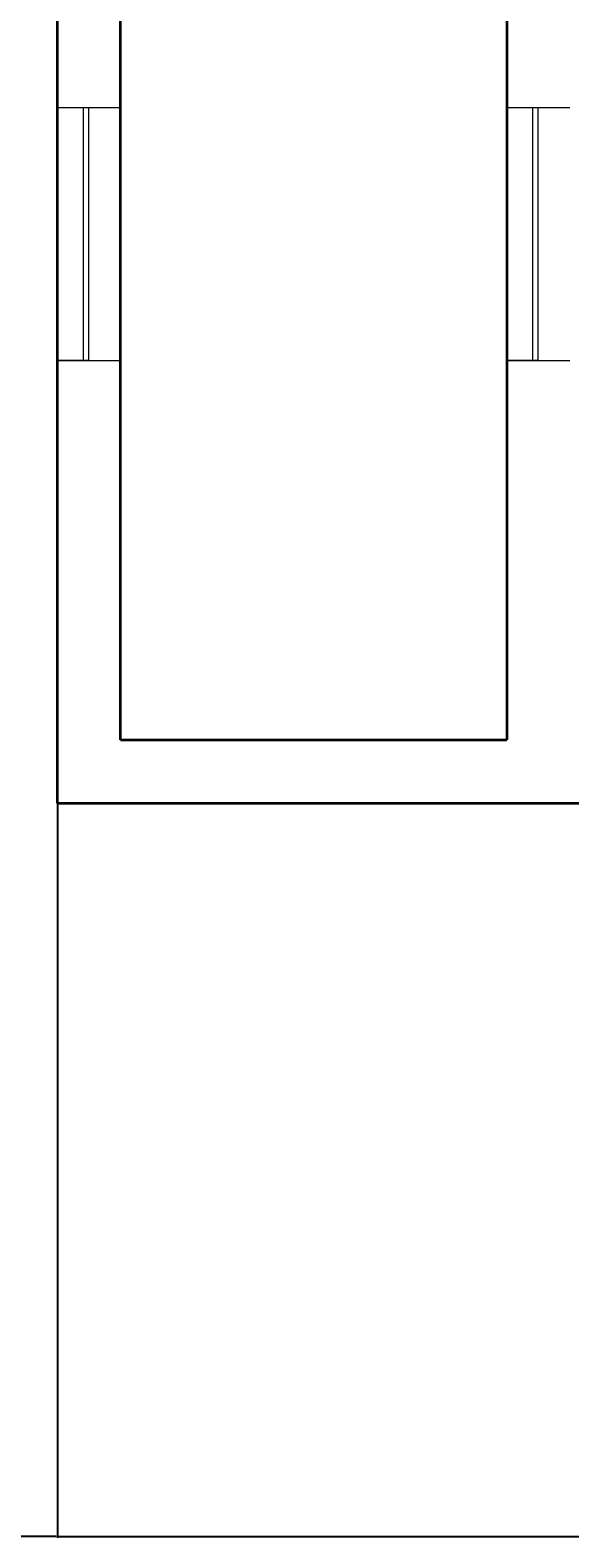
# Model space of a CAD drawing. Units: inches. Extents: x -61 to 1599, y -1316 to 257.
# Tile 156 of 204: x 989 to 1066, y -1316 to -1101. Entities that reach past the tile are written whole.
import ezdxf

# ---------------------------------------------------------------- set-up
doc = ezdxf.new("R2010")
doc.units = ezdxf.units.IN
doc.header["$MEASUREMENT"] = 0
for name, color, linetype, lineweight in [('A-ANNO-DIMS', 2, 'Continuous', 18), ('WALLS', 4, 'Continuous', 35), ('WINDOWS', 220, 'Continuous', 18)]:
    doc.layers.add(name, color=color, linetype=linetype, lineweight=lineweight)
doc.styles.get("Standard").update_dxf_attribs({"font": 'arial.ttf'})
doc.dimstyles.get("Standard").update_dxf_attribs({"dimtxt": 0.18, "dimasz": 0.18, "dimexe": 0.18, "dimexo": 0.0625, "dimgap": 0.09, "dimtad": 0, "dimtih": 1, "dimtoh": 1, "dimdec": 0, "dimzin": 0, "dimdsep": 46, "dimlunit": 3, "dimtxsty": 'Standard', "dimcen": 0.09, "dimadec": 0, "dimazin": 0, "dimtfac": 1, "dimtdec": 0, "dimtofl": 0, "dimtmove": 0, "dimatfit": 3, "dimfxl": 1, "dimtolj": 1, "dimtzin": 0, "dimarcsym": 0})

# ---------------------------------------------------------------- blocks, each defined once
blk = doc.blocks.new('WIN-36IN')
for p, q in [((0, 4.5), (0, 9)), ((0, 9), (0, 0)), ((36, 9), (36, 0)), ((0, 5.26), (36, 5.26)), ((0, 4.5), (36, 4.5)), ((0, 4.5), (36, 4.5))]:
    blk.add_line(p, q)
blk = doc.blocks.new('*D689')
at = {"layer": 'A-ANNO-DIMS', "color": 0, "lineweight": -2, "transparency": 16777216}
for p, q in [((992.7, -1211.23), (992.7, -1315.72)), ((544.7, -1216.01), (544.7, -1315.72)), ((544.88, -1315.54), (768.41, -1315.54)), ((992.52, -1315.54), (769, -1315.54))]:
    blk.add_line(p, q, dxfattribs=at)
at = {"layer": 'A-ANNO-DIMS', "color": 0, "transparency": 16777216}
for points in [[(544.88, -1315.51), (544.88, -1315.57), (544.7, -1315.54)], [(992.52, -1315.51), (992.52, -1315.57), (992.7, -1315.54)]]:
    blk.add_solid(points, dxfattribs=at)
at = {"layer": 'DEFPOINTS', "color": 0, "transparency": 16777216}
for p in [(992.7, -1211.17), (544.7, -1215.94), (992.7, -1315.54)]:
    blk.add_point(p, dxfattribs=at)
at = {"layer": 'A-ANNO-DIMS', "color": 0, "transparency": 16777216, "insert": (768.7, -1315.54), "char_height": 0.18, "attachment_point": 5}
blk.add_mtext('\\A1;448', dxfattribs=at)
blk = doc.blocks.new('*D690')
at = {"layer": 'A-ANNO-DIMS', "color": 0, "lineweight": -2, "transparency": 16777216}
for p, q in [((992.7, -1211.23), (992.7, -1315.72)), ((1522.7, -1211.23), (1522.7, -1315.72)), ((992.88, -1315.54), (1257.41, -1315.54)), ((1522.52, -1315.54), (1257.99, -1315.54))]:
    blk.add_line(p, q, dxfattribs=at)
at = {"layer": 'A-ANNO-DIMS', "color": 0, "transparency": 16777216}
for points in [[(992.88, -1315.51), (992.88, -1315.57), (992.7, -1315.54)], [(1522.52, -1315.51), (1522.52, -1315.57), (1522.7, -1315.54)]]:
    blk.add_solid(points, dxfattribs=at)
at = {"layer": 'DEFPOINTS', "color": 0, "transparency": 16777216}
for p in [(992.7, -1211.17), (1522.7, -1211.17), (1522.7, -1315.54)]:
    blk.add_point(p, dxfattribs=at)
at = {"layer": 'A-ANNO-DIMS', "color": 0, "transparency": 16777216, "insert": (1257.7, -1315.54), "char_height": 0.18, "attachment_point": 5}
blk.add_mtext('\\A1;530', dxfattribs=at)

msp = doc.modelspace()

# ---------------------------------------------------------------- linework, layer by layer
at = {"layer": 'WALLS'}
for p, q in [((992.7028, -1211.169), (992.7028, -741.169)), ((1001.7028, -1202.169), (1001.7028, -777.169)), ((1056.7028, -945.169), (1056.7028, -1202.169)), ((1001.7028, -1202.169), (1056.7028, -1202.169)), ((992.7028, -1211.169), (1215.7028, -1211.169))]:
    msp.add_line(p, q, dxfattribs=at)

# ---------------------------------------------------------------- block references
at = {"layer": 'WINDOWS'}
for p, rotation in [((1001.7029, -1148.1651), 89.99999999999969), ((1065.7029, -1148.1651), 89.99999999999939)]:
    msp.add_blockref('WIN-36IN', p, dxfattribs=dict(at, rotation=rotation))

# ---------------------------------------------------------------- dimensions: what is measured, and where the dimension line sits
at = {"layer": 'A-ANNO-DIMS'}
for base, p1, p2, picture, middle in [((992.7028, -1315.5446), (544.7028, -1215.9446), (992.7028, -1211.169), '*D689', (768.7028, -1315.5446)), ((1522.7028, -1315.5446), (992.7028, -1211.169), (1522.7028, -1211.169), '*D690', (1257.7028, -1315.5446))]:
    dim = msp.add_linear_dim(base=base, p1=p1, p2=p2, dimstyle='Standard', override={"dimdec": 0, "dimlfac": 1, "dimrnd": 0, "dimzin": 0, "dimdsep": 46, "dimlunit": 2}, dxfattribs=at)
    dim.commit()
    dim.dimension.update_dxf_attribs({"geometry": picture, "text_midpoint": middle})

doc.saveas('drawing.dxf')
